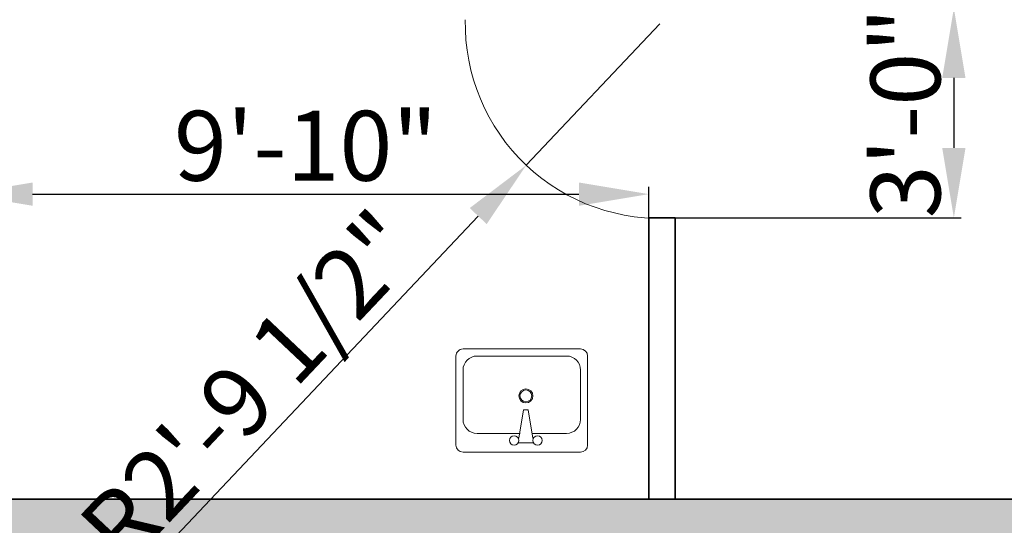
# Model space of a CAD drawing. Units: inches. Extents: x 2083 to 3317, y 1141 to 2115.
# Tile 92 of 256: x 2246 to 2415, y 1707 to 1794. Entities that reach past the tile are written whole.
import ezdxf

# ---------------------------------------------------------------- set-up
doc = ezdxf.new("R2010")
doc.units = ezdxf.units.IN
for name, color, linetype, lineweight in [('A-ANNO-DIMS', 2, 'Continuous', 18), ('A-DOOR', 4, 'Continuous', 18), ('A-FLOR-FIXT', 9, 'Continuous', 18), ('A-WALL', 7, 'Continuous', 35)]:
    doc.layers.add(name, color=color, linetype=linetype, lineweight=lineweight)
doc.layers.add('A-WALL-PATT', color=251, linetype='Continuous', lineweight=13, true_color=0x636466)
doc.styles.add('DIM_FONT', font='TXT.shx', dxfattribs={"width": 0.8})
doc.styles.get("Standard").update_dxf_attribs({"font": 'arial.ttf'})
doc.dimstyles.new('ISO-25', dxfattribs={"dimtxt": 12, "dimasz": 12, "dimexe": 1.25, "dimexo": 0.625, "dimtad": 1, "dimlunit": 3, "dimtxsty": 'Standard', "dimcen": 2.5, "dimadec": 0, "dimazin": 0, "dimtfac": 1, "dimtmove": 0, "dimatfit": 3, "dimfxl": 1, "dimarcsym": 0})

# ---------------------------------------------------------------- blocks, each defined once
blk = doc.blocks.new('A$C564A496C')
at = {"linetype": 'ByBlock'}
for p, q in [((543.2, 450), (30.7, 450)), ((0, 419.3), (0, 30.7)), ((238.5, 409.1), (299.8, 409.1)), ((238.5, 388.6), (258.9, 265.9)), ((279.4, 265.9), (299.8, 388.6)), ((573.8, 30.7), (573.8, 419.3)), ((92, 368.2), (243.6, 368.2)), ((294.7, 368.2), (481.8, 368.2)), ((30.7, 92), (30.7, 306.8)), ((543.2, 306.8), (543.2, 92)), ((258.9, 265.9), (279.4, 265.9)), ((30.7, 0), (543.2, 0)), ((481.8, 30.7), (92, 30.7))]:
    blk.add_line(p, q, dxfattribs=at)
for centre, radius in [((218, 398.9), 20.5), ((320.3, 398.9), 20.5), ((269.1, 204.5), 30.7), ((269.1, 204.5), 25.7)]:
    blk.add_circle(centre, radius, dxfattribs=at)
for centre, radius, start, end in [((30.7, 419.3), 30.7, 90, 180), ((543.2, 419.3), 30.7, 0, 90), ((92, 306.8), 61.4, 90, 180), ((481.8, 306.8), 61.4, 0, 90), ((92, 92), 61.4, 180, 270), ((481.8, 92), 61.4, 270, 0), ((30.7, 30.7), 30.7, 180, 270), ((543.2, 30.7), 30.7, 270, 0)]:
    blk.add_arc(centre, radius, start, end, dxfattribs=at)
at = {"style": 'DIM_FONT', "width": 0.8, "flags": 9}
for tag in ['YSIZE', 'XSIZE']:
    blk.add_attdef(tag, (269.1, 450), '', height=0.5, rotation=270, dxfattribs=at)
blk = doc.blocks.new('*D40')
at = {"layer": 'A-ANNO-DIMS', "color": 0, "lineweight": -2, "transparency": 16777216}
for p, q in [((2235.96, 1712.39), (2235.96, 1765.36)), ((2353.71, 1712.39), (2353.71, 1765.36)), ((2247.96, 1764.11), (2341.71, 1764.11))]:
    blk.add_line(p, q, dxfattribs=at)
at = {"layer": 'A-ANNO-DIMS', "color": 0, "transparency": 16777216}
for points in [[(2247.96, 1766.11), (2247.96, 1762.11), (2235.96, 1764.11)], [(2341.71, 1766.11), (2341.71, 1762.11), (2353.71, 1764.11)]]:
    blk.add_solid(points, dxfattribs=at)
at = {"layer": 'Defpoints', "color": 0, "transparency": 16777216}
for p in [(2353.71, 1764.11), (2235.96, 1711.76), (2353.71, 1711.76)]:
    blk.add_point(p, dxfattribs=at)
at = {"layer": 'A-ANNO-DIMS', "color": 0, "transparency": 16777216, "insert": (2294.83, 1770.86), "char_height": 12, "attachment_point": 5}
blk.add_mtext('9\'-10"', dxfattribs=at)
blk = doc.blocks.new('*D56')
at = {"layer": 'A-ANNO-DIMS', "color": 0, "lineweight": -2, "transparency": 16777216}
for p, q in [((2354.33, 1796.05), (2407.31, 1796.05)), ((2406.06, 1784.05), (2406.06, 1772.05)), ((2354.33, 1760.05), (2407.31, 1760.05))]:
    blk.add_line(p, q, dxfattribs=at)
at = {"layer": 'A-ANNO-DIMS', "color": 0, "transparency": 16777216}
for points in [[(2404.06, 1784.05), (2408.06, 1784.05), (2406.06, 1796.05)], [(2404.06, 1772.05), (2408.06, 1772.05), (2406.06, 1760.05)]]:
    blk.add_solid(points, dxfattribs=at)
at = {"layer": 'Defpoints', "color": 0, "transparency": 16777216}
for p in [(2353.71, 1796.05), (2353.71, 1760.05), (2406.06, 1760.05)]:
    blk.add_point(p, dxfattribs=at)
at = {"layer": 'A-ANNO-DIMS', "color": 0, "transparency": 16777216, "insert": (2399.3, 1778.05), "char_height": 12, "attachment_point": 5, "rotation": 90}
blk.add_mtext('3\'-0"', dxfattribs=at)
blk = doc.blocks.new('*D69')
at = {"layer": 'A-ANNO-DIMS', "color": 0, "lineweight": -2, "transparency": 16777216}
for p, q in [((2355.6, 1793.35), (2332.67, 1769.07)), ((2266.34, 1698.84), (2324.43, 1760.34))]:
    blk.add_line(p, q, dxfattribs=at)
at = {"layer": 'A-ANNO-DIMS', "color": 0, "transparency": 16777216}
blk.add_solid([(2322.97, 1761.72), (2325.88, 1758.97), (2332.67, 1769.07)], dxfattribs=at)
at = {"layer": 'Defpoints', "color": 0, "transparency": 16777216}
for p in [(2355.6, 1793.35), (2332.67, 1769.07)]:
    blk.add_point(p, dxfattribs=at)
at = {"layer": 'A-ANNO-DIMS', "color": 0, "transparency": 16777216, "insert": (2286.3, 1729.92), "char_height": 12, "attachment_point": 5, "rotation": 46.6362}
blk.add_mtext('R2\'-9 1/2"', dxfattribs=at)

msp = doc.modelspace()

# ---------------------------------------------------------------- hatches: boundary and pattern name
at = {"layer": 'A-WALL-PATT'}
h = msp.add_hatch(color=256, dxfattribs=at)
h.dxf.hatch_style = 1
h.paths.add_polyline_path([(3126.96, 2020.761), (2748.96, 2020.761), (2604.96, 2020.761), (2226.96, 2020.761), (2226.96, 1702.761), (2466.96, 1702.761), (2466.96, 1582.761), (2418.96, 1582.761), (2418.96, 1477.761), (2226.96, 1477.761), (2226.96, 1263.261), (2544.96, 1263.261), (2544.96, 1411.761), (2604.96, 1411.761), (2685.96, 1411.761), (2685.96, 1420.761), (2604.96, 1420.761), (2604.96, 1573.761), (2604.96, 1702.761), (2604.96, 2011.761), (2748.96, 2011.761), (2748.96, 1702.761), (2862.96, 1702.761), (2862.96, 1621.761), (2871.96, 1621.761), (2871.96, 1702.761), (2883.96, 1702.761), (2883.96, 1706.939, -0.0264593), (2883.96, 1711.761), (2757.96, 1711.761), (2757.96, 1807.761), (2787.96, 1807.761), (2787.96, 1812.261), (2757.96, 1812.261), (2757.96, 2011.761), (2877.96, 2011.761), (2877.96, 1812.261), (2847.96, 1812.261), (2847.96, 1807.761), (2889.836, 1807.761), (2889.836, 1812.261), (2882.46, 1812.261), (2882.46, 2011.761), (3117.96, 2011.761), (3117.96, 1812.261), (2937.836, 1812.261), (2937.836, 1807.761), (2995.71, 1807.761), (2995.71, 1796.118), (3000.21, 1796.118), (3000.21, 1807.761), (3117.96, 1807.761), (3117.96, 1711.761), (3000.21, 1711.761), (3000.21, 1760.118), (2998.573, 1760.118, -0.020711), (2995.71, 1760.118), (2995.71, 1711.761), (2931.96, 1711.761), (2931.96, 1702.761), (3126.96, 1702.761)])
h.paths.add_polyline_path([(2471.46, 2011.761), (2471.46, 1810.011), (2462.717, 1810.011), (2462.717, 1805.511), (2505.96, 1805.511), (2505.96, 1810.011), (2475.96, 1810.011), (2475.96, 2011.761), (2595.96, 2011.761), (2595.96, 1810.011), (2565.96, 1810.011), (2565.96, 1805.511), (2595.96, 1805.511), (2595.96, 1711.761), (2235.96, 1711.761), (2235.96, 1805.511), (2353.71, 1805.511), (2353.71, 1796.054), (2358.21, 1796.054), (2358.21, 1805.511), (2414.717, 1805.511), (2414.717, 1810.011), (2235.96, 1810.011), (2235.96, 2011.761)], flags=16)
h.paths.add_polyline_path([(2270.205, 1994.61), (2270.205, 1970.61), (2246.205, 1970.61), (2246.205, 1994.61)], flags=0)
edge = h.paths.add_edge_path(flags=0)
edge.add_ellipse((2332.027, 1899.798), major_axis=(-3.043, 3.043), ratio=0.1682525, start_angle=-161.33217, end_angle=-156.30711, ccw=False)
edge.add_ellipse((2333.082, 1898.744), major_axis=(-1.055, 1.055), ratio=0.4535321, start_angle=-123.37102, end_angle=-94.15911)
edge = h.paths.add_edge_path(flags=0)
edge.add_ellipse((2332.027, 1968.876), major_axis=(3.043, 3.043), ratio=0.1682525, start_angle=18.66783, end_angle=23.69289)
edge.add_spline(control_points=[(2332.926, 1970.691), (2332.227, 1970.336), (2330.894, 1969.659), (2328.413, 1970.932), (2327.204, 1967.749), (2324.71, 1969.956), (2322.533, 1967.012), (2320.013, 1971.296), (2317.68, 1968.158), (2316.041, 1967.102), (2315.427, 1966.81)], knot_values=[0, 0, 0, 0, 2.2670587, 4.3245589, 6.6855835, 8.8786411, 11.121502, 14.300359, 17.7552837, 19.732645, 19.732645, 19.732645, 19.732645], degree=3, periodic=0)
edge.add_ellipse((2332.027, 1968.876), major_axis=(3.043, 3.043), ratio=0.1682525, start_angle=18.66783, end_angle=23.69289, ccw=False)
edge.add_ellipse((2333.082, 1969.931), major_axis=(1.055, 1.055), ratio=0.4535321, start_angle=56.62898, end_angle=85.84089, ccw=False)
edge = h.paths.add_edge_path(flags=0)
edge.add_spline(control_points=[(2296.428, 1967.988), (2293.628, 1965.336), (2287.704, 1959.727), (2299.744, 1949.996), (2294.533, 1935.669), (2290.573, 1920.604), (2293.394, 1909.974), (2296.185, 1904.967)], knot_values=[0.0991853, 0.0991853, 0.0991853, 0.0991853, 0.3453009, 0.6198217, 0.9826526, 1.3860932, 1.8105546, 1.8105546, 1.8105546, 1.8105546], degree=3, periodic=0)
edge.add_spline(control_points=[(2296.185, 1904.967), (2297.384, 1902.619), (2298.001, 1901.949), (2298.553, 1901.468)], knot_values=[0.0062457, 0.0062457, 0.0062457, 0.0062457, 0.0554759, 0.0554759, 0.0554759, 0.0554759], degree=3, periodic=0)
edge.add_spline(control_points=[(2298.553, 1901.468), (2297.259, 1900.923), (2295.225, 1900.232), (2293.06, 1900.614), (2292.101, 1900.788), (2292.09, 1900.791)], knot_values=[0.3128349, 0.3128349, 0.3128349, 0.3128349, 0.4017797, 0.4749867, 0.4759027, 0.4759027, 0.4759027, 0.4759027], degree=3, periodic=0)
edge.add_arc((2292.794, 1904.664), 3.937, 215.4209, 259.69818, ccw=False)
edge.add_spline(control_points=[(2289.585, 1902.382), (2289.477, 1902.535), (2289.368, 1902.688), (2289.261, 1902.841)], knot_values=[0.1028719, 0.1028719, 0.1028719, 0.1028719, 0.1168958, 0.1168958, 0.1168958, 0.1168958], degree=3, periodic=0)
edge.add_spline(control_points=[(2289.261, 1902.841), (2288.687, 1902.55), (2287.64, 1902.02), (2285.881, 1901.874), (2283.853, 1901.504), (2281.72, 1899.711), (2278.467, 1899.493), (2276.157, 1901.883), (2272.259, 1899.804), (2267.778, 1901.843), (2262.244, 1900.184), (2257.415, 1901.782), (2254.318, 1900.726), (2253.178, 1900.337)], knot_values=[0, 0, 0, 0, 1.9079767, 3.4771759, 5.261074, 7.9728515, 11.6802485, 13.7179214, 16.9395917, 22.789562, 27.5025027, 33.5952153, 37.1456181, 37.1456181, 37.1456181, 37.1456181], degree=3, periodic=0)
edge.add_line((2253.178, 1900.337), (2250.244, 1902.841))
edge.add_line((2250.244, 1902.841), (2250.244, 1965.833))
edge.add_line((2250.244, 1965.833), (2253.178, 1968.337))
edge.add_spline(control_points=[(2253.178, 1968.337), (2254.318, 1967.948), (2257.415, 1966.892), (2262.244, 1968.49), (2267.778, 1966.831), (2271.527, 1968.537), (2273.876, 1967.828), (2274.207, 1967.728)], knot_values=[0, 0, 0, 0, 0.0901802, 0.2449351, 0.3646438, 0.5132331, 0.5378548, 0.5378548, 0.5378548, 0.5378548], degree=3, periodic=0)
edge.add_arc((2274.353, 1963.793), 3.937, 72.05113, 92.12795, ccw=False)
edge.add_arc((2281.297, 1985.23), 18.596, 252.05113, 288.56572)
edge.add_arc((2292.317, 1956.029), 12.646, 71.02679, 113.77822, ccw=False)
edge = h.paths.add_edge_path(flags=0)
edge.add_spline(control_points=[(2274.899, 1951.856), (2275.066, 1951.617), (2275.233, 1951.377), (2275.398, 1951.136)], knot_values=[1.4099157, 1.4099157, 1.4099157, 1.4099157, 1.4315903, 1.4315903, 1.4315903, 1.4315903], degree=3, periodic=0)
edge.add_spline(control_points=[(2275.398, 1951.136), (2275.792, 1950.562), (2276.179, 1949.984), (2276.546, 1949.397)], knot_values=[1.3582378, 1.3582378, 1.3582378, 1.3582378, 1.4099157, 1.4099157, 1.4099157, 1.4099157], degree=3, periodic=0)
edge.add_line((2276.546, 1949.397), (2277.437, 1947.862))
edge.add_spline(control_points=[(2277.437, 1947.862), (2276.304, 1945.673), (2274.64, 1942.427), (2274.632, 1938.094), (2272.799, 1930.852), (2274.356, 1943.897), (2275.948, 1947.923), (2276.546, 1949.397)], knot_values=[0.0056315, 0.0056315, 0.0056315, 0.0056315, 0.1860139, 0.2660015, 0.3570872, 0.5963902, 0.7397317, 0.7397317, 0.7397317, 0.7397317], degree=3, periodic=0)
edge.add_spline(control_points=[(2276.546, 1949.397), (2276.179, 1949.984), (2275.792, 1950.562), (2275.398, 1951.136)], knot_values=[1.3582378, 1.3582378, 1.3582378, 1.3582378, 1.4099157, 1.4099157, 1.4099157, 1.4099157], degree=3, periodic=0)
edge.add_spline(control_points=[(2275.398, 1951.136), (2274.943, 1950.08), (2274.208, 1948.025), (2273.935, 1944.851), (2272.469, 1937.627), (2273.466, 1945.696), (2274.701, 1951.059), (2274.899, 1951.856)], knot_values=[0.1043639, 0.1043639, 0.1043639, 0.1043639, 0.1896363, 0.2696239, 0.3607096, 0.6000126, 0.6446217, 0.6446217, 0.6446217, 0.6446217], degree=3, periodic=0)
h.paths.add_polyline_path([(2269.168, 1963.128, -0.3575267), (2268.171, 1960.976, -0.0925607), (2268.171, 1939.436, -0.3575267), (2269.168, 1937.285, -0.3575267), (2267.016, 1938.282, -0.1647847), (2254.686, 1938.282, -0.3575267), (2252.534, 1937.285, -0.3575267), (2253.531, 1939.436, -0.0925607), (2253.531, 1960.976, -0.3575267), (2252.534, 1963.128, -0.3575267), (2254.686, 1962.131, -0.1647847), (2267.016, 1962.131, -0.3575267)], flags=0)
h.paths.add_polyline_path([(2248.874, 1967.802), (2248.874, 1957.028), (2249.458, 1957.028), (2249.458, 1911.647), (2248.874, 1911.647), (2248.874, 1900.873), (2246.512, 1900.873, 0.1973271), (2244.15, 1902.457), (2244.15, 1966.218, 0.1973271), (2246.512, 1967.802)], flags=0)
h.paths.add_polyline_path([(2269.168, 1931.389, -0.3575267), (2268.171, 1929.238, -0.0925607), (2268.171, 1907.698, -0.3575267), (2269.168, 1905.547, -0.3575267), (2267.016, 1906.544, -0.1647847), (2254.686, 1906.544, -0.3575267), (2252.534, 1905.547, -0.3575267), (2253.531, 1907.698, -0.0925607), (2253.531, 1929.238, -0.3575267), (2252.534, 1931.389, -0.3575267), (2254.686, 1930.392, -0.1647847), (2267.016, 1930.392, -0.3575267)], flags=0)
edge = h.paths.add_edge_path(flags=0)
edge.add_spline(control_points=[(2276.197, 1906.724), (2276.168, 1909.029), (2276.114, 1913.372), (2270.598, 1924.925), (2273.905, 1919.013), (2275.922, 1916.262), (2275.475, 1912.402), (2277.258, 1910.381), (2276.696, 1908.225), (2276.646, 1906.813), (2276.618, 1906.008)], knot_values=[0, 0, 0, 0, 8.6102597, 16.2212739, 18.8430575, 23.8048978, 27.4408283, 29.3561016, 31.2034776, 33.6506866, 33.6506866, 33.6506866, 33.6506866], degree=3, periodic=0)
edge.add_spline(control_points=[(2276.618, 1906.008), (2276.623, 1905.624), (2276.498, 1904.629), (2275.442, 1903.855), (2274.937, 1903.08), (2274.859, 1902.841)], knot_values=[0.1564884, 0.1564884, 0.1564884, 0.1564884, 0.1843975, 0.2313765, 0.2505985, 0.2505985, 0.2505985, 0.2505985], degree=3, periodic=0)
edge.add_line((2274.859, 1902.841), (2276.506, 1902.841))
edge.add_spline(control_points=[(2276.506, 1902.841), (2276.788, 1903.085), (2277.665, 1904.125), (2278.25, 1904.341), (2277.654, 1908.527), (2278.156, 1906.228), (2278.1, 1905.286), (2278.847, 1904.069), (2277.857, 1903.415), (2277.874, 1902.991), (2277.904, 1902.841)], knot_values=[0.0595743, 0.0595743, 0.0595743, 0.0595743, 0.0807529, 0.1037415, 0.1697201, 0.1760361, 0.2071372, 0.2404744, 0.2623409, 0.2736605, 0.2736605, 0.2736605, 0.2736605], degree=3, periodic=0)
edge.add_line((2277.904, 1902.841), (2280.03, 1902.841))
edge.add_spline(control_points=[(2280.03, 1902.841), (2279.888, 1903.088), (2279.499, 1903.982), (2280.152, 1905.939), (2278.104, 1909.658), (2279.762, 1907.185), (2280.328, 1904.875), (2280.485, 1903.49), (2281.463, 1903.249), (2281.758, 1902.936), (2281.834, 1902.841)], knot_values=[0.013856, 0.013856, 0.013856, 0.013856, 0.0348738, 0.0888667, 0.1078792, 0.1267378, 0.158714, 0.1937575, 0.2174868, 0.2267221, 0.2267221, 0.2267221, 0.2267221], degree=3, periodic=0)
edge.add_spline(control_points=[(2281.834, 1902.841), (2281.788, 1902.827), (2281.647, 1902.783), (2281.396, 1902.859), (2281.088, 1902.985), (2280.721, 1903.061), (2280.333, 1903.026), (2280.125, 1902.899), (2280.03, 1902.841)], knot_values=[0, 0, 0, 0, 0.1441304, 0.435517, 0.7492759, 1.1530457, 1.5483707, 1.878348, 1.878348, 1.878348, 1.878348], degree=3, periodic=0)
edge.add_line((2280.03, 1902.841), (2277.904, 1902.841))
edge.add_spline(control_points=[(2277.904, 1902.841), (2277.893, 1902.796), (2277.865, 1902.68), (2277.607, 1902.687), (2277.274, 1902.801), (2276.838, 1902.62), (2276.584, 1902.789), (2276.506, 1902.841)], knot_values=[0, 0, 0, 0, 0.1271885, 0.3261988, 0.6280094, 1.2435704, 1.5153306, 1.5153306, 1.5153306, 1.5153306], degree=3, periodic=0)
edge.add_line((2276.506, 1902.841), (2274.859, 1902.841))
edge.add_spline(control_points=[(2274.859, 1902.841), (2274.814, 1902.899), (2274.725, 1903.013), (2274.493, 1903.119), (2274.244, 1902.961), (2273.937, 1903.185), (2273.614, 1902.983), (2273.408, 1902.883), (2273.322, 1902.841)], knot_values=[0, 0, 0, 0, 0.2184302, 0.4369566, 0.6879766, 0.9903786, 1.3983955, 1.6918498, 1.6918498, 1.6918498, 1.6918498], degree=3, periodic=0)
edge.add_spline(control_points=[(2273.322, 1902.841), (2273.617, 1903.446), (2274.274, 1904.538), (2276.027, 1904.574), (2276.207, 1906.584), (2276.197, 1906.724)], knot_values=[0.0122268, 0.0122268, 0.0122268, 0.0122268, 0.0594721, 0.1062177, 0.134458, 0.134458, 0.134458, 0.134458], degree=3, periodic=0)
h.paths.add_polyline_path([(2270.776, 1897.79), (2270.776, 1873.79), (2246.776, 1873.79), (2246.776, 1897.79)], flags=0)
h.paths.add_polyline_path([(2353.71, 1760.005), (2353.71, 1760.054), (2358.21, 1760.054, -0.033729)], flags=0)
h.paths.add_polyline_path([(2321.819, 1737.529), (2341.995, 1737.529, -0.4142136), (2343.203, 1736.321), (2343.203, 1721.021, -0.4142136), (2341.995, 1719.813), (2321.819, 1719.813, -0.4142136), (2320.611, 1721.021), (2320.611, 1736.321, -0.4142136)], flags=0)
h.paths.add_polyline_path([(2324.235, 1736.321), (2339.579, 1736.321, -0.4142136), (2341.995, 1733.905), (2341.995, 1725.45, -0.4142136), (2339.579, 1723.034), (2333.681, 1723.034), (2333.845, 1722.045, -0.8706461), (2335.425, 1721.826, -0.767327), (2333.923, 1721.423), (2331.291, 1721.423, -0.767327), (2329.788, 1721.826, -0.8706461), (2331.368, 1722.045), (2331.533, 1723.034), (2324.235, 1723.034, -0.4142136), (2321.819, 1725.45), (2321.819, 1733.905, -0.4142136)], flags=0)
h.paths.add_polyline_path([(2570.484, 1928.615), (2589.684, 1928.615), (2590.169, 1928.615), (2590.169, 1904.993), (2570.484, 1904.993)], flags=0)
h.paths.add_polyline_path([(2574.447, 1927.264, -1), (2572.829, 1927.264, -1)], flags=0)
h.paths.add_polyline_path([(2573.09, 1926.941), (2573.925, 1927.776), (2574.148, 1927.553), (2573.313, 1926.718)], flags=0)
h.paths.add_polyline_path([(2578.779, 1919.73, -1), (2571.592, 1919.73, -1)], flags=0)
h.paths.add_polyline_path([(2578.385, 1919.73, -1), (2571.985, 1919.73, -1)], flags=0)
h.paths.add_polyline_path([(2331.596, 1729.476, -1), (2333.618, 1729.476, -1)], flags=0)
h.paths.add_polyline_path([(2578.034, 1927.264, -1), (2576.416, 1927.264, -1)], flags=0)
h.paths.add_polyline_path([(2576.689, 1927.531), (2576.912, 1927.754), (2577.747, 1926.919), (2577.524, 1926.696)], flags=0)
h.paths.add_polyline_path([(2578.139, 1909.86, -1), (2572.232, 1909.86, -1)], flags=0)
h.paths.add_polyline_path([(2577.745, 1909.86, -1), (2572.625, 1909.86, -1)], flags=0)
h.paths.add_polyline_path([(2583.798, 1927.264, -1), (2582.179, 1927.264, -1)], flags=0)
h.paths.add_polyline_path([(2582.719, 1927.754), (2583.554, 1926.919), (2583.331, 1926.696), (2582.496, 1927.531)], flags=0)
h.paths.add_polyline_path([(2582.496, 1927.531), (2582.719, 1927.754), (2583.554, 1926.919), (2583.331, 1926.696)], flags=0)
h.paths.add_polyline_path([(2587.739, 1920.53, -1), (2581.832, 1920.53, -1)], flags=0)
h.paths.add_polyline_path([(2587.345, 1920.53, -1), (2582.225, 1920.53, -1)], flags=0)
h.paths.add_polyline_path([(2587.385, 1927.264, -1), (2585.766, 1927.264, -1)], flags=0)
h.paths.add_polyline_path([(2586.082, 1926.98), (2586.917, 1927.815), (2587.14, 1927.593), (2586.305, 1926.758)], flags=0)
h.paths.add_polyline_path([(2588.379, 1910.66, -1), (2581.192, 1910.66, -1)], flags=0)
h.paths.add_polyline_path([(2587.985, 1910.66, -1), (2581.585, 1910.66, -1)], flags=0)
h.paths.add_polyline_path([(2417.168, 1729.478), (2437.344, 1729.478, -0.4142136), (2438.552, 1728.27), (2438.552, 1712.969, -0.4142136), (2437.344, 1711.761), (2417.168, 1711.761, -0.4142136), (2415.96, 1712.969), (2415.96, 1728.27, -0.4142136)], flags=0)
h.paths.add_polyline_path([(2419.584, 1728.27), (2434.928, 1728.27, -0.4142136), (2437.344, 1725.854), (2437.344, 1717.398, -0.4142136), (2434.928, 1714.983), (2429.029, 1714.983), (2429.194, 1713.994, -0.8706461), (2430.774, 1713.775, -0.767327), (2429.271, 1713.372), (2426.64, 1713.372, -0.767327), (2425.137, 1713.775, -0.8706461), (2426.717, 1713.994), (2426.882, 1714.983), (2419.584, 1714.983, -0.4142136), (2417.168, 1717.398), (2417.168, 1725.854, -0.4142136)], flags=0)
h.paths.add_polyline_path([(2419.584, 1728.27), (2434.928, 1728.27, -0.4142136), (2437.344, 1725.854), (2437.344, 1717.398, -0.4142136), (2434.928, 1714.983), (2429.029, 1714.983), (2428.358, 1719.009), (2427.553, 1719.009), (2426.882, 1714.983), (2419.584, 1714.983, -0.4142136), (2417.168, 1717.398), (2417.168, 1725.854, -0.4142136)], flags=0)
h.paths.add_polyline_path([(2426.944, 1721.425, -1), (2428.967, 1721.425, -1)], flags=0)
h.paths.add_polyline_path([(2475.96, 1702.761), (2595.96, 1702.761), (2595.96, 1582.761), (2475.96, 1582.761)], flags=16)
h.paths.add_polyline_path([(2427.96, 1573.761), (2595.96, 1573.761), (2595.96, 1468.761), (2595.96, 1420.761), (2384.46, 1420.761), (2384.46, 1468.761), (2427.96, 1468.761)], flags=16)
h.paths.add_polyline_path([(2379.96, 1468.761), (2379.96, 1420.761), (2235.96, 1420.761), (2235.96, 1468.761)], flags=16)
h.paths.add_polyline_path([(2317.816, 1466.696), (2337.992, 1466.696, -0.4142136), (2339.2, 1465.488), (2339.2, 1450.187, -0.4142136), (2337.992, 1448.979), (2317.816, 1448.979, -0.4142136), (2316.608, 1450.187), (2316.608, 1465.488, -0.4142136)], flags=0)
h.paths.add_polyline_path([(2320.232, 1465.488), (2335.576, 1465.488, -0.4142136), (2337.992, 1463.072), (2337.992, 1454.616, -0.4142136), (2335.576, 1452.2), (2329.677, 1452.2), (2329.842, 1451.212, -0.8706461), (2331.422, 1450.992, -0.767327), (2329.92, 1450.59), (2327.288, 1450.59, -0.767327), (2325.785, 1450.992, -0.8706461), (2327.365, 1451.212), (2327.53, 1452.2), (2320.232, 1452.2, -0.4142136), (2317.816, 1454.616), (2317.816, 1463.072, -0.4142136)], flags=0)
h.paths.add_polyline_path([(2320.232, 1465.488), (2335.576, 1465.488, -0.4142136), (2337.992, 1463.072), (2337.992, 1454.616, -0.4142136), (2335.576, 1452.2), (2329.677, 1452.2), (2329.006, 1456.227), (2328.201, 1456.227), (2327.53, 1452.2), (2320.232, 1452.2, -0.4142136), (2317.816, 1454.616), (2317.816, 1463.072, -0.4142136)], flags=0)
h.paths.add_polyline_path([(2327.593, 1458.643, -1), (2329.615, 1458.643, -1)], flags=0)
h.paths.add_polyline_path([(2244.412, 1433.34), (2241.921, 1433.34, -0.4142136), (2240.018, 1435.244), (2240.018, 1440.953, -0.4142105), (2241.921, 1442.856), (2244.412, 1442.856, -1.9764724)], flags=0)
h.paths.add_polyline_path([(2245.357, 1434.398, -0.4142136), (2245.357, 1441.799, -2.1440985)], flags=0)
h.paths.add_polyline_path([(2535.96, 1416.261), (2535.96, 1272.261), (2235.96, 1272.261), (2235.96, 1416.261)], flags=16)
h.paths.add_polyline_path([(2260.12, 1384.293), (2260.12, 1362.039), (2237.865, 1362.039), (2237.865, 1384.293)], flags=0)
edge = h.paths.add_edge_path(flags=0)
edge.add_line((2318.252, 1362.093), (2318.146, 1362.001))
edge.add_ellipse((2317.445, 1360.431), major_axis=(2.822, 2.822), ratio=0.1682525, start_angle=18.66783, end_angle=20.94813, ccw=False)
edge.add_ellipse((2318.423, 1361.409), major_axis=(0.978, 0.978), ratio=0.4535321, start_angle=56.62898, end_angle=70.2262, ccw=False)
edge = h.paths.add_edge_path(flags=0)
edge.add_line((2319.107, 1295.571), (2319.015, 1295.677))
edge.add_ellipse((2317.445, 1296.378), major_axis=(-2.822, 2.822), ratio=0.1682525, start_angle=-161.33217, end_angle=-159.05187, ccw=False)
edge.add_ellipse((2318.423, 1295.4), major_axis=(-0.978, 0.978), ratio=0.4535321, start_angle=-123.37102, end_angle=-109.7738)
edge = h.paths.add_edge_path(flags=0)
edge.add_spline(control_points=[(2284.21, 1301.17), (2284.581, 1300.445), (2284.891, 1299.892), (2285.16, 1299.461)], knot_values=[0.0390658, 0.0390658, 0.0390658, 0.0390658, 0.0554759, 0.0554759, 0.0554759, 0.0554759], degree=3, periodic=0)
edge.add_line((2285.16, 1299.461), (2284.21, 1301.17))
edge = h.paths.add_edge_path(flags=0)
edge.add_line((2280.412, 1297.298), (2283.37, 1297.036))
edge.add_line((2283.37, 1297.036), (2286.406, 1297.926))
edge.add_spline(control_points=[(2286.406, 1297.926), (2285.305, 1297.463), (2284.345, 1297.129), (2283.37, 1297.036)], knot_values=[0.3943688, 0.3943688, 0.3943688, 0.3943688, 0.4759027, 0.4759027, 0.4759027, 0.4759027], degree=3, periodic=0)
edge.add_spline(control_points=[(2283.37, 1297.036), (2283.281, 1297.028), (2282.316, 1296.957), (2281.313, 1297.134), (2280.423, 1297.296), (2280.412, 1297.298)], knot_values=[0.3128349, 0.3128349, 0.3128349, 0.3128349, 0.3202458, 0.3934528, 0.3943688, 0.3943688, 0.3943688, 0.3943688], degree=3, periodic=0)
edge = h.paths.add_edge_path(flags=0)
edge.add_line((2284.436, 1359.607), (2280.446, 1355.328))
edge.add_line((2280.446, 1355.328), (2279.58, 1351.018))
edge.add_line((2279.58, 1351.018), (2282.413, 1346.58))
edge.add_spline(control_points=[(2282.413, 1346.58), (2283.153, 1345.589), (2284.253, 1344.029), (2284.801, 1342.387), (2284.935, 1341.806)], knot_values=[1.2400982, 1.2400982, 1.2400982, 1.2400982, 1.3328922, 1.3827123, 1.3827123, 1.3827123, 1.3827123], degree=3, periodic=0)
edge.add_spline(control_points=[(2284.935, 1341.806), (2285.319, 1340.141), (2285.233, 1338.409), (2284.91, 1336.654)], knot_values=[1.0974841, 1.0974841, 1.0974841, 1.0974841, 1.2400982, 1.2400982, 1.2400982, 1.2400982], degree=3, periodic=0)
edge.add_spline(control_points=[(2284.91, 1336.654), (2284.587, 1334.899), (2284.027, 1333.12), (2283.463, 1331.361)], knot_values=[0.9548699, 0.9548699, 0.9548699, 0.9548699, 1.0974841, 1.0974841, 1.0974841, 1.0974841], degree=3, periodic=0)
edge.add_line((2283.463, 1331.361), (2281.89, 1326.153))
edge.add_line((2281.89, 1326.153), (2280.756, 1321.056))
edge.add_line((2280.756, 1321.056), (2280.299, 1316.002))
edge.add_line((2280.299, 1316.002), (2280.716, 1310.95))
edge.add_line((2280.716, 1310.95), (2282.028, 1305.972))
edge.add_line((2282.028, 1305.972), (2284.21, 1301.17))
edge.add_spline(control_points=[(2284.21, 1301.17), (2283.341, 1302.73), (2282.612, 1304.336), (2282.028, 1305.972)], knot_values=[0.0991853, 0.0991853, 0.0991853, 0.0991853, 0.2417994, 0.2417994, 0.2417994, 0.2417994], degree=3, periodic=0)
edge.add_spline(control_points=[(2282.028, 1305.972), (2281.444, 1307.608), (2281.005, 1309.273), (2280.716, 1310.95)], knot_values=[0.2417994, 0.2417994, 0.2417994, 0.2417994, 0.3844135, 0.3844135, 0.3844135, 0.3844135], degree=3, periodic=0)
edge.add_spline(control_points=[(2280.716, 1310.95), (2280.433, 1312.588), (2280.289, 1314.277), (2280.299, 1315.962), (2280.299, 1316.002)], knot_values=[0.3844135, 0.3844135, 0.3844135, 0.3844135, 0.5236467, 0.5270276, 0.5270276, 0.5270276, 0.5270276], degree=3, periodic=0)
edge.add_spline(control_points=[(2280.299, 1316.002), (2280.312, 1317.687), (2280.478, 1319.368), (2280.756, 1321.056)], knot_values=[0.5270276, 0.5270276, 0.5270276, 0.5270276, 0.6696417, 0.6696417, 0.6696417, 0.6696417], degree=3, periodic=0)
edge.add_spline(control_points=[(2280.756, 1321.056), (2281.035, 1322.744), (2281.426, 1324.44), (2281.89, 1326.153)], knot_values=[0.6696417, 0.6696417, 0.6696417, 0.6696417, 0.8122558, 0.8122558, 0.8122558, 0.8122558], degree=3, periodic=0)
edge.add_spline(control_points=[(2281.89, 1326.153), (2282.264, 1327.533), (2282.788, 1329.262), (2283.353, 1331.018), (2283.463, 1331.361)], knot_values=[0.8122558, 0.8122558, 0.8122558, 0.8122558, 0.9270873, 0.9548699, 0.9548699, 0.9548699, 0.9548699], degree=3, periodic=0)
edge.add_line((2283.463, 1331.361), (2284.91, 1336.654))
edge.add_line((2284.91, 1336.654), (2284.935, 1341.806))
edge.add_line((2284.935, 1341.806), (2282.413, 1346.58))
edge.add_spline(control_points=[(2282.413, 1346.58), (2281.275, 1348.104), (2280.078, 1349.57), (2279.58, 1351.018)], knot_values=[1.3827123, 1.3827123, 1.3827123, 1.3827123, 1.5253264, 1.5253264, 1.5253264, 1.5253264], degree=3, periodic=0)
edge.add_spline(control_points=[(2279.58, 1351.018), (2279.443, 1351.415), (2279.136, 1352.857), (2279.735, 1354.29), (2280.446, 1355.328)], knot_values=[1.5253264, 1.5253264, 1.5253264, 1.5253264, 1.564439, 1.6679405, 1.6679405, 1.6679405, 1.6679405], degree=3, periodic=0)
edge.add_spline(control_points=[(2280.446, 1355.328), (2281.426, 1356.758), (2282.931, 1358.183), (2284.436, 1359.607)], knot_values=[1.6679405, 1.6679405, 1.6679405, 1.6679405, 1.8105546, 1.8105546, 1.8105546, 1.8105546], degree=3, periodic=0)
edge.add_arc((2280.623, 1348.518), 11.726, 71.02679, 113.77822)
edge.add_arc((2270.405, 1375.595), 17.244, 252.05113, 288.56572, ccw=False)
edge.add_arc((2263.966, 1355.718), 3.651, 72.05113, 92.12795)
edge.add_arc((2263.966, 1355.718), 3.651, 92.12795, 177.98513)
edge.add_spline(control_points=[(2260.318, 1355.846), (2260.26, 1354.221), (2260.551, 1350.187), (2262.999, 1346.766), (2264.473, 1344.649)], knot_values=[1.4315903, 1.4315903, 1.4315903, 1.4315903, 1.5641438, 1.7706953, 1.7706953, 1.7706953, 1.7706953], degree=3, periodic=0)
edge.add_line((2264.473, 1344.649), (2264.936, 1343.983))
edge.add_spline(control_points=[(2263.801, 1340.248), (2263.843, 1340.514), (2264.067, 1341.756), (2264.513, 1343.002), (2264.935, 1343.981)], knot_values=[0.5365702, 0.5365702, 0.5365702, 0.5365702, 0.5593494, 0.6446217, 0.6446217, 0.6446217, 0.6446217], degree=3, periodic=0)
edge.add_spline(control_points=[(2264.935, 1343.981), (2265.118, 1343.715), (2265.299, 1343.448), (2265.477, 1343.179)], knot_values=[1.3840767, 1.3840767, 1.3840767, 1.3840767, 1.4099157, 1.4099157, 1.4099157, 1.4099157], degree=3, periodic=0)
edge.add_spline(control_points=[(2265.477, 1343.179), (2265.655, 1342.911), (2265.829, 1342.641), (2265.999, 1342.369)], knot_values=[1.3582378, 1.3582378, 1.3582378, 1.3582378, 1.3840767, 1.3840767, 1.3840767, 1.3840767], degree=3, periodic=0)
edge.add_line((2265.999, 1342.369), (2266.826, 1340.946))
edge.add_spline(control_points=[(2266.826, 1340.946), (2268.894, 1337.09), (2271.398, 1325.843), (2270.516, 1310.569), (2275.919, 1301.861), (2277.79, 1299.199)], knot_values=[0.1168958, 0.1168958, 0.1168958, 0.1168958, 0.4729873, 1.0509689, 1.3137934, 1.3137934, 1.3137934, 1.3137934], degree=3, periodic=0)
edge.add_spline(control_points=[(2277.79, 1299.199), (2277.839, 1299.128), (2277.889, 1299.057), (2277.94, 1298.987)], knot_values=[0.1098839, 0.1098839, 0.1098839, 0.1098839, 0.1168958, 0.1168958, 0.1168958, 0.1168958], degree=3, periodic=0)
edge.add_line((2277.94, 1298.987), (2277.789, 1299.199))
edge.add_spline(control_points=[(2277.789, 1299.199), (2277.257, 1298.929), (2276.286, 1298.438), (2275.039, 1298.334), (2274.383, 1298.239), (2274.215, 1298.209)], knot_values=[33.1218702, 33.1218702, 33.1218702, 33.1218702, 35.0290557, 36.5982549, 37.1448269, 37.1448269, 37.1448269, 37.1448269], degree=3, periodic=0)
edge.add_line((2274.215, 1298.209), (2273.073, 1297.893))
edge.add_spline(control_points=[(2273.073, 1297.893), (2272.323, 1297.58), (2271.039, 1296.511), (2269.248, 1296.226), (2268.423, 1296.375)], knot_values=[26.5325843, 26.5325843, 26.5325843, 26.5325843, 29.198919, 31.8391012, 31.8391012, 31.8391012, 31.8391012], degree=3, periodic=0)
edge.add_line((2268.423, 1296.375), (2263.879, 1297.458))
edge.add_spline(control_points=[(2263.879, 1297.458), (2263.556, 1297.359), (2261.86, 1296.839), (2260.239, 1297.282), (2258.933, 1297.516)], knot_values=[15.9195506, 15.9195506, 15.9195506, 15.9195506, 16.9395917, 21.2260675, 21.2260675, 21.2260675, 21.2260675], degree=3, periodic=0)
edge.add_line((2258.933, 1297.516), (2254.055, 1297.329))
edge.add_spline(control_points=[(2254.055, 1297.329), (2253.756, 1297.296), (2252.114, 1297.165), (2250.462, 1297.544), (2249.13, 1297.668)], knot_values=[5.3065169, 5.3065169, 5.3065169, 5.3065169, 6.2764352, 10.6130337, 10.6130337, 10.6130337, 10.6130337], degree=3, periodic=0)
edge.add_line((2249.13, 1297.668), (2244.332, 1296.878))
edge.add_line((2244.332, 1296.878), (2241.611, 1299.199))
edge.add_line((2241.611, 1299.199), (2241.611, 1357.609))
edge.add_line((2241.611, 1357.609), (2244.332, 1359.931))
edge.add_line((2244.332, 1359.931), (2252.729, 1359.543))
edge.add_spline(control_points=[(2252.729, 1359.543), (2252.871, 1359.546), (2253.306, 1359.548), (2253.74, 1359.514), (2254.032, 1359.482)], knot_values=[0.233291, 0.233291, 0.233291, 0.233291, 0.2449351, 0.2689274, 0.2689274, 0.2689274, 0.2689274], degree=3, periodic=0)
edge.add_line((2254.032, 1359.482), (2259.587, 1359.416))
edge.add_spline(control_points=[(2259.587, 1359.416), (2260.677, 1359.629), (2262.073, 1359.897), (2263.524, 1359.459), (2263.83, 1359.366)], knot_values=[0.4225164, 0.4225164, 0.4225164, 0.4225164, 0.5132331, 0.5378548, 0.5378548, 0.5378548, 0.5378548], degree=3, periodic=0)
edge.add_arc((2263.966, 1355.718), 3.651, 72.05113, 92.12795, ccw=False)
edge.add_arc((2270.405, 1375.595), 17.244, 252.05113, 288.56572)
edge.add_arc((2280.623, 1348.518), 11.726, 71.02679, 113.77822, ccw=False)
h.paths.add_polyline_path([(2240.341, 1359.435), (2240.341, 1349.444), (2240.882, 1349.444), (2240.882, 1307.365), (2240.341, 1307.365), (2240.341, 1297.374), (2238.15, 1297.374, 0.1973271), (2235.96, 1298.843), (2235.96, 1357.966, 0.1973271), (2238.15, 1359.435)], flags=0)
h.paths.add_polyline_path([(2259.158, 1355.101, -0.3575267), (2258.233, 1353.106, -0.0925607), (2258.233, 1333.133, -0.3575267), (2259.158, 1331.138, -0.3575267), (2257.163, 1332.062, -0.1647847), (2245.729, 1332.062, -0.3575267), (2243.735, 1331.138, -0.3575267), (2244.659, 1333.133, -0.0925607), (2244.659, 1353.106, -0.3575267), (2243.735, 1355.101, -0.3575267), (2245.729, 1354.176, -0.1647847), (2257.163, 1354.176, -0.3575267)], flags=0)
edge = h.paths.add_edge_path(flags=0)
edge.add_line((2265.999, 1342.369), (2266.826, 1340.946))
edge.add_line((2266.826, 1340.946), (2265.308, 1337.814))
edge.add_line((2265.308, 1337.814), (2264.358, 1334.653))
edge.add_line((2264.358, 1334.653), (2264.262, 1333.8))
edge.add_spline(control_points=[(2264.262, 1333.8), (2264.208, 1333.187), (2264.162, 1332.366), (2264.007, 1331.414), (2263.969, 1331.202)], knot_values=[0.4644442, 0.4644442, 0.4644442, 0.4644442, 0.5166905, 0.5316081, 0.5316081, 0.5316081, 0.5316081], degree=3, periodic=0)
edge.add_spline(control_points=[(2263.969, 1331.202), (2263.775, 1330.119), (2263.424, 1328.791), (2263.257, 1328.531), (2263.234, 1328.515)], knot_values=[0.3726816, 0.3726816, 0.3726816, 0.3726816, 0.4488497, 0.4644442, 0.4644442, 0.4644442, 0.4644442], degree=3, periodic=0)
edge.add_spline(control_points=[(2263.234, 1328.515), (2263.096, 1328.42), (2263.131, 1329.301), (2263.275, 1330.616)], knot_values=[0.2809191, 0.2809191, 0.2809191, 0.2809191, 0.3726816, 0.3726816, 0.3726816, 0.3726816], degree=3, periodic=0)
edge.add_spline(control_points=[(2263.275, 1330.616), (2263.419, 1331.93), (2263.672, 1333.677), (2263.97, 1335.315)], knot_values=[0.1891566, 0.1891566, 0.1891566, 0.1891566, 0.2809191, 0.2809191, 0.2809191, 0.2809191], degree=3, periodic=0)
edge.add_spline(control_points=[(2263.97, 1335.315), (2264.1, 1336.032), (2264.419, 1337.622), (2264.755, 1338.864), (2264.947, 1339.491)], knot_values=[0.097394, 0.097394, 0.097394, 0.097394, 0.1375775, 0.1891566, 0.1891566, 0.1891566, 0.1891566], degree=3, periodic=0)
edge.add_spline(control_points=[(2264.947, 1339.491), (2265.29, 1340.606), (2265.644, 1341.494), (2265.999, 1342.369)], knot_values=[0.0056315, 0.0056315, 0.0056315, 0.0056315, 0.097394, 0.097394, 0.097394, 0.097394], degree=3, periodic=0)
h.paths.add_polyline_path([(2259.158, 1325.671, -0.3575267), (2258.233, 1323.676, -0.0925607), (2258.233, 1303.703, -0.3575267), (2259.158, 1301.708, -0.3575267), (2257.163, 1302.633, -0.1647847), (2245.729, 1302.633, -0.3575267), (2243.735, 1301.708, -0.3575267), (2244.659, 1303.703, -0.0925607), (2244.659, 1323.676, -0.3575267), (2243.735, 1325.671, -0.3575267), (2245.729, 1324.747, -0.1647847), (2257.163, 1324.747, -0.3575267)], flags=0)
edge = h.paths.add_edge_path(flags=0)
edge.add_spline(control_points=[(2261.709, 1317.311), (2261.679, 1317.418), (2261.762, 1317.389), (2262.491, 1316.09), (2262.962, 1315.301)], knot_values=[14.9558607, 14.9558607, 14.9558607, 14.9558607, 16.2212739, 18.6948259, 18.6948259, 18.6948259, 18.6948259], degree=3, periodic=0)
edge.add_spline(control_points=[(2262.962, 1315.301), (2262.99, 1315.254), (2263.702, 1314.067), (2264.349, 1313.127), (2264.73, 1312.164)], knot_values=[18.6948259, 18.6948259, 18.6948259, 18.6948259, 18.8430575, 22.433791, 22.433791, 22.433791, 22.433791], degree=3, periodic=0)
edge.add_spline(control_points=[(2264.73, 1312.164), (2264.876, 1311.796), (2265.177, 1310.77), (2265.143, 1309.559), (2265.248, 1308.824)], knot_values=[22.433791, 22.433791, 22.433791, 22.433791, 23.8048978, 26.1727562, 26.1727562, 26.1727562, 26.1727562], degree=3, periodic=0)
edge.add_line((2265.248, 1308.824), (2265.851, 1307.172))
edge.add_spline(control_points=[(2265.851, 1307.172), (2266.065, 1306.822), (2266.384, 1306.332), (2266.424, 1305.781), (2266.42, 1305.611)], knot_values=[28.0625624, 28.0625624, 28.0625624, 28.0625624, 29.3561016, 29.9117214, 29.9117214, 29.9117214, 29.9117214], degree=3, periodic=0)
edge.add_spline(control_points=[(2266.42, 1305.611), (2266.416, 1305.433), (2266.394, 1305.25), (2266.365, 1305.066)], knot_values=[29.9117214, 29.9117214, 29.9117214, 29.9117214, 30.4978371, 30.4978371, 30.4978371, 30.4978371], degree=3, periodic=0)
edge.add_line((2266.365, 1305.066), (2266.066, 1302.136))
edge.add_spline(control_points=[(2266.066, 1302.136), (2266.071, 1301.78), (2265.998, 1301.2), (2265.663, 1300.759), (2265.509, 1300.586)], knot_values=[0.1564884, 0.1564884, 0.1564884, 0.1564884, 0.1843975, 0.2035434, 0.2035434, 0.2035434, 0.2035434], degree=3, periodic=0)
edge.add_line((2265.509, 1300.586), (2264.435, 1299.199))
edge.add_line((2264.435, 1299.199), (2265.962, 1299.199))
edge.add_line((2265.962, 1299.199), (2267.336, 1301.175))
edge.add_line((2267.336, 1301.175), (2267.312, 1301.986))
edge.add_spline(control_points=[(2267.312, 1301.986), (2267.261, 1302.862), (2267.16, 1303.737), (2267.271, 1303.326)], knot_values=[0.1262286, 0.1262286, 0.1262286, 0.1262286, 0.1666174, 0.1666174, 0.1666174, 0.1666174], degree=3, periodic=0)
edge.add_spline(control_points=[(2267.271, 1303.326), (2267.28, 1303.294), (2267.31, 1303.175), (2267.373, 1302.884), (2267.406, 1302.683), (2267.418, 1302.601)], knot_values=[0.1666174, 0.1666174, 0.1666174, 0.1666174, 0.1697201, 0.1760361, 0.1807647, 0.1807647, 0.1807647, 0.1807647], degree=3, periodic=0)
edge.add_spline(control_points=[(2267.744, 1300.988), (2267.688, 1301.151), (2267.481, 1301.657), (2267.484, 1302.145), (2267.418, 1302.601)], knot_values=[0.1807647, 0.1807647, 0.1807647, 0.1807647, 0.1937665, 0.2201389, 0.2201389, 0.2201389, 0.2201389], degree=3, periodic=0)
edge.add_line((2267.418, 1302.601), (2267.744, 1300.988))
edge.add_spline(control_points=[(2267.744, 1300.988), (2267.832, 1300.732), (2267.932, 1300.31), (2267.555, 1299.975), (2267.429, 1299.829)], knot_values=[0.2201389, 0.2201389, 0.2201389, 0.2201389, 0.2404744, 0.2548903, 0.2548903, 0.2548903, 0.2548903], degree=3, periodic=0)
edge.add_line((2267.429, 1299.829), (2267.258, 1299.199))
edge.add_line((2267.258, 1299.199), (2269.23, 1299.199))
edge.add_spline(control_points=[(2269.23, 1299.199), (2269.099, 1299.429), (2268.843, 1300.016), (2269.012, 1300.916), (2268.947, 1301.661)], knot_values=[0.013856, 0.013856, 0.013856, 0.013856, 0.0348738, 0.0670726, 0.0670726, 0.0670726, 0.0670726], degree=3, periodic=0)
edge.add_line((2268.947, 1301.661), (2268.432, 1303.603))
edge.add_spline(control_points=[(2268.432, 1303.603), (2268.176, 1304.192), (2267.596, 1305.251), (2268.041, 1304.623), (2268.251, 1304.282)], knot_values=[0.0901547, 0.0901547, 0.0901547, 0.0901547, 0.1078792, 0.1202891, 0.1202891, 0.1202891, 0.1202891], degree=3, periodic=0)
edge.add_spline(control_points=[(2268.251, 1304.282), (2268.361, 1304.105), (2269.058, 1302.918), (2269.383, 1301.59), (2269.521, 1300.776), (2269.575, 1300.556)], knot_values=[0.1202891, 0.1202891, 0.1202891, 0.1202891, 0.1267378, 0.158714, 0.1735056, 0.1735056, 0.1735056, 0.1735056], degree=3, periodic=0)
edge.add_line((2269.575, 1300.556), (2270.686, 1299.421))
edge.add_spline(control_points=[(2270.686, 1299.421), (2270.767, 1299.357), (2270.838, 1299.281), (2270.903, 1299.199)], knot_values=[0.2181597, 0.2181597, 0.2181597, 0.2181597, 0.2267221, 0.2267221, 0.2267221, 0.2267221], degree=3, periodic=0)
edge.add_line((2270.937, 1299.193), (2270.903, 1299.199))
edge.add_spline(control_points=[(2270.903, 1299.199), (2270.86, 1299.186), (2270.73, 1299.146), (2270.496, 1299.216), (2270.272, 1299.308), (2270.121, 1299.348), (2270.063, 1299.36)], knot_values=[0.939174, 0.939174, 0.939174, 0.939174, 1.0833044, 1.3746911, 1.6884499, 1.878348, 1.878348, 1.878348, 1.878348], degree=3, periodic=0)
edge.add_line((2270.063, 1299.36), (2269.23, 1299.199))
edge.add_line((2269.23, 1299.199), (2267.258, 1299.199))
edge.add_spline(control_points=[(2267.258, 1299.199), (2267.248, 1299.157), (2267.223, 1299.05), (2266.984, 1299.057), (2266.809, 1299.116), (2266.677, 1299.109), (2266.637, 1299.105)], knot_values=[0.7576653, 0.7576653, 0.7576653, 0.7576653, 0.8848538, 1.0838641, 1.3856747, 1.5153306, 1.5153306, 1.5153306, 1.5153306], degree=3, periodic=0)
edge.add_spline(control_points=[(2266.637, 1299.105), (2266.485, 1299.089), (2266.236, 1299.017), (2266.035, 1299.151), (2265.962, 1299.199)], knot_values=[0, 0, 0, 0, 0.4859051, 0.7576653, 0.7576653, 0.7576653, 0.7576653], degree=3, periodic=0)
edge.add_line((2265.962, 1299.199), (2264.435, 1299.199))
edge.add_line((2264.435, 1299.199), (2263.858, 1299.367))
edge.add_spline(control_points=[(2263.858, 1299.367), (2263.819, 1299.371), (2263.78, 1299.386), (2263.74, 1299.402)], knot_values=[0.8459249, 0.8459249, 0.8459249, 0.8459249, 0.9786272, 0.9786272, 0.9786272, 0.9786272], degree=3, periodic=0)
edge.add_line((2263.722, 1299.396), (2263.01, 1299.199))
edge.add_spline(control_points=[(2263.01, 1299.199), (2263.246, 1299.683), (2263.506, 1300.128), (2263.873, 1300.408)], knot_values=[0.0122268, 0.0122268, 0.0122268, 0.0122268, 0.0529705, 0.0529705, 0.0529705, 0.0529705], degree=3, periodic=0)
edge.add_spline(control_points=[(2263.873, 1300.408), (2263.932, 1300.453), (2264.084, 1300.553), (2264.255, 1300.624), (2264.36, 1300.665)], knot_values=[0.0529705, 0.0529705, 0.0529705, 0.0529705, 0.0594721, 0.0690861, 0.0690861, 0.0690861, 0.0690861], degree=3, periodic=0)
edge.add_line((2264.36, 1300.665), (2265.142, 1301.078))
edge.add_line((2265.142, 1301.078), (2265.676, 1302.8))
edge.add_line((2265.676, 1302.8), (2265.541, 1305.704))
edge.add_line((2265.541, 1305.704), (2264.803, 1309.328))
edge.add_line((2264.803, 1309.328), (2263.041, 1314.092))
edge.add_spline(control_points=[(2263.041, 1314.092), (2262.384, 1315.671), (2261.796, 1316.998), (2261.709, 1317.311)], knot_values=[11.2168955, 11.2168955, 11.2168955, 11.2168955, 14.9558607, 14.9558607, 14.9558607, 14.9558607], degree=3, periodic=0)
h.paths.add_polyline_path([(2871.96, 1416.261), (2895.91, 1416.261), (2895.91, 1420.761), (2871.96, 1420.761), (2871.96, 1501.761), (2862.96, 1501.761), (2862.96, 1420.761), (2805.96, 1420.761), (2805.96, 1411.761), (2862.96, 1411.761), (2862.96, 1263.261), (3126.96, 1263.261), (3126.96, 1411.761), (3126.96, 1486.761), (2943.96, 1486.761), (2943.96, 1477.761), (2967.86, 1477.761), (2967.86, 1420.761), (2943.91, 1420.761), (2943.91, 1416.261), (3117.96, 1416.261), (3117.96, 1420.761), (2972.36, 1420.761), (2972.36, 1477.761), (3117.96, 1477.761), (3117.96, 1420.761), (3117.96, 1272.261), (2871.96, 1272.261)], flags=0)
h.paths.add_polyline_path([(2457.126, 1485.943), (2527.603, 1485.943), (2527.603, 1537.636), (2457.126, 1537.636)], flags=8)
h.paths.add_polyline_path([(2481.005, 1609.982), (2590.766, 1609.982), (2590.766, 1682.003), (2481.005, 1682.003)], flags=8)
h.paths.add_polyline_path([(2483.085, 1729.127), (2553.562, 1729.127), (2553.562, 1780.82), (2483.085, 1780.82)], flags=8)

# ---------------------------------------------------------------- linework, layer by layer
at = {"layer": 'A-DOOR'}
msp.add_arc((2355.596, 1793.346), 33.394, 178.78438, 274.48877, dxfattribs=at)
at = {"layer": 'A-WALL'}
for p, q in [((2353.71, 1760.054), (2358.21, 1760.054)), ((2353.71, 1760.054), (2353.71, 1711.761)), ((2358.21, 1760.054), (2358.21, 1711.761)), ((2235.96, 1711.761), (2595.96, 1711.761))]:
    msp.add_line(p, q, dxfattribs=at)

# ---------------------------------------------------------------- block references
at = {"layer": 'A-FLOR-FIXT', "xscale": 0.0393700787401575, "yscale": 0.0393700787401575, "zscale": 0.0393700787401575, "rotation": 180}
msp.add_blockref('A$C564A496C', (2343.203, 1737.529), dxfattribs=at)

# ---------------------------------------------------------------- dimensions: what is measured, and where the dimension line sits
at = {"layer": 'A-ANNO-DIMS'}
dim = msp.add_linear_dim(base=(2406.06, 1760.054), p1=(2353.71, 1796.054), p2=(2353.71, 1760.054), angle=270, dimstyle='ISO-25', override={"dimdec": 1, "dimlfac": 1, "dimrnd": 0, "dimzin": 1, "dimdsep": 46, "dimlunit": 4, "dimfrac": 2}, dxfattribs=at)
dim.commit()
dim.dimension.update_dxf_attribs({"geometry": '*D56', "text_midpoint": (2399.304, 1778.054)})
dim = msp.add_radius_dim(center=(2355.596, 1793.346), mpoint=(2332.667, 1769.068), dimstyle='ISO-25', override={"dimdec": 1, "dimlfac": 1, "dimrnd": 0, "dimzin": 1, "dimdsep": 46, "dimlunit": 4, "dimfrac": 2}, dxfattribs=at)
dim.commit()
dim.dimension.update_dxf_attribs({"geometry": '*D69', "text_midpoint": (2286.3, 1729.921)})
dim = msp.add_linear_dim(base=(2353.709783, 1764.11136), p1=(2235.959783, 1711.76136), p2=(2353.709783, 1711.76136), dimstyle='ISO-25', override={"dimdec": 1, "dimlfac": 1, "dimrnd": 0, "dimzin": 1, "dimdsep": 46, "dimlunit": 4, "dimfrac": 2}, dxfattribs=at)
dim.commit()
dim.dimension.update_dxf_attribs({"geometry": '*D40', "text_midpoint": (2294.834783, 1770.863235853)})

doc.saveas('drawing.dxf')
